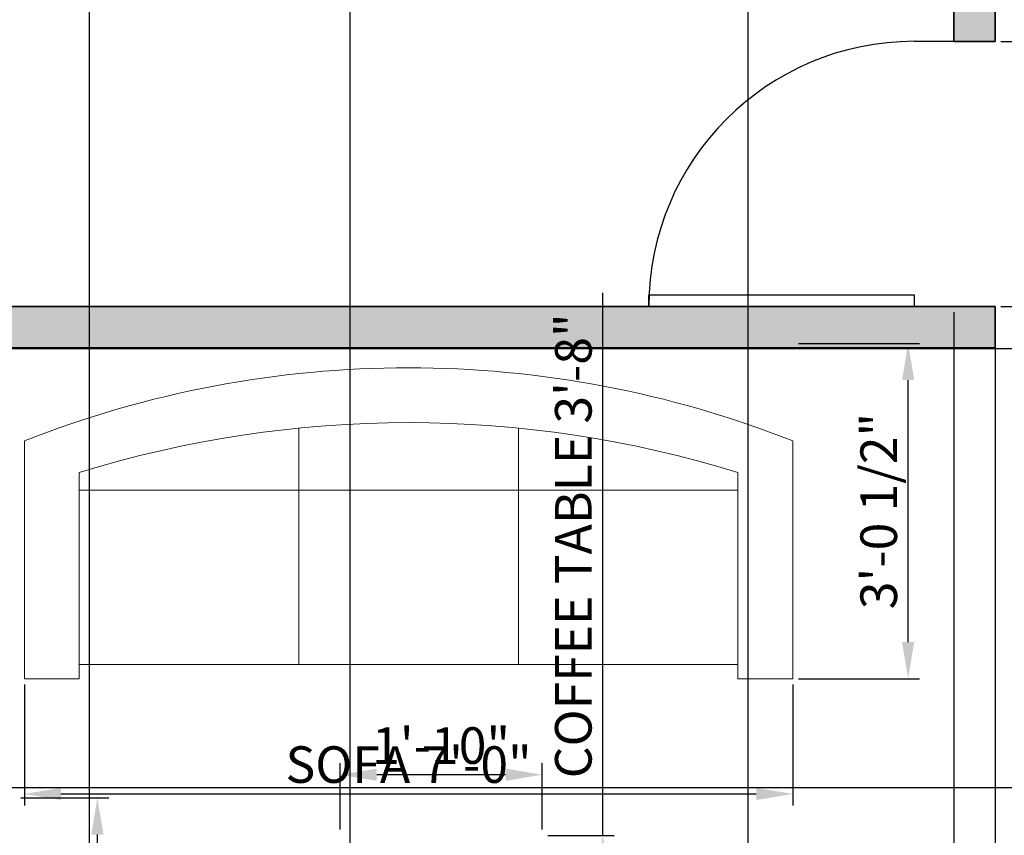
# Model space of a CAD drawing. Units: inches. Extents: x 1872 to 2380, y 714 to 1327.
# Tile 6 of 9: x 1994 to 2101, y 1055 to 1144. Entities that reach past the tile are written whole.
import ezdxf

# ---------------------------------------------------------------- set-up
doc = ezdxf.new("R2010")
doc.units = ezdxf.units.IN
for name, color, linetype, lineweight in [('A-ANNO-DIMS', 2, 'Continuous', 18), ('A-DOOR', 4, 'Continuous', 25), ('A-FURN', 8, 'Continuous', 18), ('A-WALL', 7, 'Continuous', 35)]:
    doc.layers.add(name, color=color, linetype=linetype, lineweight=lineweight)
doc.layers.add('A-WALL-PATT', color=242, linetype='Continuous', lineweight=13, true_color=0xd52e31)
doc.styles.get("Standard").update_dxf_attribs({"font": 'arial.ttf'})
doc.dimstyles.new('ISO-25', dxfattribs={"dimtxt": 4, "dimasz": 4, "dimexe": 1.25, "dimexo": 0.625, "dimtad": 1, "dimdec": 0, "dimlunit": 3, "dimtxsty": 'Standard', "dimcen": 2.5, "dimadec": 0, "dimazin": 0, "dimtfac": 1, "dimtdec": 0, "dimtmove": 0, "dimatfit": 3, "dimfxl": 1, "dimarcsym": 0})

# ---------------------------------------------------------------- blocks, each defined once
blk = doc.blocks.new('*U3')
for p, q in [((0, 0), (0, -6)), ((40, 0), (40, -6))]:
    blk.add_line(p, q)
blk.add_lwpolyline([(0, 0), (0, 40), (1.75, 40), (1.75, 0)], close=True)
blk.add_arc((0, 0), 40, 0, 90)
blk = doc.blocks.new('Sofa - Roundback 7 ft.')
for p, q in [((-12.00002, -32.4421), (-12.00003, -6.5971)), ((11.99997, -32.4421), (11.99998, -6.5971)), ((-36.000027, -34), (-36.000027, -11.4696)), ((35.99998, -34), (35.99998, -11.4696)), ((-35.999844, -13.3819), (35.9998, -13.3819)), ((-36.000027, -32.4421), (35.99998, -32.4421))]:
    blk.add_line(p, q)
for points in [[(-36.000027, -34), (-42.000027, -34), (-42.000027, -8)], [(41.99998, -8), (41.99998, -34), (35.99998, -34)]]:
    blk.add_lwpolyline(points)
for centre, radius, start, end in [((0, -114.25), 114.25, 68.43141, 111.5686), ((-0.00001, -127.1968), 121.1968, 72.72033, 107.2797)]:
    blk.add_arc(centre, radius, start, end)
blk = doc.blocks.new('*D40')
at = {"layer": 'A-ANNO-DIMS', "color": 0, "lineweight": -2, "transparency": 16777216}
for p, q in [((1993.9, 1059.04), (2003.52, 1059.04)), ((2002.27, 1003.04), (2002.27, 1055.04)), ((1993.9, 999.04), (2003.52, 999.04))]:
    blk.add_line(p, q, dxfattribs=at)
at = {"layer": 'A-ANNO-DIMS', "color": 0, "transparency": 16777216}
for points in [[(2001.61, 1055.04), (2002.94, 1055.04), (2002.27, 1059.04)], [(2001.61, 1003.04), (2002.94, 1003.04), (2002.27, 999.04)]]:
    blk.add_solid(points, dxfattribs=at)
at = {"layer": 'Defpoints', "color": 0, "transparency": 16777216}
for p in [(1993.27, 1059.04), (2002.27, 1059.04), (1993.27, 999.04)]:
    blk.add_point(p, dxfattribs=at)
at = {"layer": 'A-ANNO-DIMS', "color": 0, "transparency": 16777216, "insert": (1999.58, 1029.04), "char_height": 4, "attachment_point": 5, "rotation": 90}
blk.add_mtext('LOVESEAT 5\'-0"', dxfattribs=at)
blk = doc.blocks.new('*D42')
at = {"layer": 'A-ANNO-DIMS', "color": 0, "lineweight": -2, "transparency": 16777216}
for p, q in [((1994.29, 1071.45), (1994.29, 1058.23)), ((2078.29, 1071.45), (2078.29, 1058.23)), ((1998.29, 1059.48), (2074.29, 1059.48))]:
    blk.add_line(p, q, dxfattribs=at)
at = {"layer": 'A-ANNO-DIMS', "color": 0, "transparency": 16777216}
for points in [[(1998.29, 1060.14), (1998.29, 1058.81), (1994.29, 1059.48)], [(2074.29, 1060.14), (2074.29, 1058.81), (2078.29, 1059.48)]]:
    blk.add_solid(points, dxfattribs=at)
at = {"layer": 'Defpoints', "color": 0, "transparency": 16777216}
for p in [(1994.29, 1072.08), (2078.29, 1072.08), (2078.29, 1059.48)]:
    blk.add_point(p, dxfattribs=at)
at = {"layer": 'A-ANNO-DIMS', "color": 0, "transparency": 16777216, "insert": (2036.29, 1062.17), "char_height": 4, "attachment_point": 5}
blk.add_mtext('SOFA 7\'-0"', dxfattribs=at)
blk = doc.blocks.new('*D43')
at = {"layer": 'A-ANNO-DIMS', "color": 0, "lineweight": -2, "transparency": 16777216}
for p, q in [((2078.91, 1108.74), (2092.14, 1108.74)), ((2090.89, 1076.08), (2090.89, 1104.74)), ((2078.91, 1072.08), (2092.14, 1072.08))]:
    blk.add_line(p, q, dxfattribs=at)
at = {"layer": 'A-ANNO-DIMS', "color": 0, "transparency": 16777216}
for points in [[(2090.22, 1104.74), (2091.55, 1104.74), (2090.89, 1108.74)], [(2090.22, 1076.08), (2091.55, 1076.08), (2090.89, 1072.08)]]:
    blk.add_solid(points, dxfattribs=at)
at = {"layer": 'Defpoints', "color": 0, "transparency": 16777216}
for p in [(2078.29, 1108.74), (2090.89, 1108.74), (2078.29, 1072.08)]:
    blk.add_point(p, dxfattribs=at)
at = {"layer": 'A-ANNO-DIMS', "color": 0, "transparency": 16777216, "insert": (2088.19, 1090.41), "char_height": 4, "attachment_point": 5, "rotation": 90}
blk.add_mtext('3\'-0 1/2"', dxfattribs=at)
blk = doc.blocks.new('*D44')
at = {"layer": 'A-ANNO-DIMS', "color": 0, "lineweight": -2, "transparency": 16777216}
for p, q in [((2057.51, 1054.95), (2057.51, 1114.26)), ((2051.51, 1054.95), (2058.76, 1054.95)), ((2057.51, 1014.78), (2057.51, 1050.95)), ((2051.51, 1010.78), (2058.76, 1010.78))]:
    blk.add_line(p, q, dxfattribs=at)
at = {"layer": 'A-ANNO-DIMS', "color": 0, "transparency": 16777216}
for points in [[(2056.84, 1050.95), (2058.17, 1050.95), (2057.51, 1054.95)], [(2056.84, 1014.78), (2058.17, 1014.78), (2057.51, 1010.78)]]:
    blk.add_solid(points, dxfattribs=at)
at = {"layer": 'Defpoints', "color": 0, "transparency": 16777216}
for p in [(2050.88, 1054.95), (2057.51, 1054.95), (2050.88, 1010.78)]:
    blk.add_point(p, dxfattribs=at)
at = {"layer": 'A-ANNO-DIMS', "color": 0, "transparency": 16777216, "insert": (2054.81, 1086.61), "char_height": 4, "attachment_point": 5, "rotation": 90}
blk.add_mtext('COFFEE TABLE 3\'-8"', dxfattribs=at)
blk = doc.blocks.new('*D45')
at = {"layer": 'A-ANNO-DIMS', "color": 0, "lineweight": -2, "transparency": 16777216}
for p, q in [((2028.8, 1055.58), (2028.8, 1062.83)), ((2050.88, 1055.58), (2050.88, 1062.83)), ((2046.88, 1061.58), (2032.8, 1061.58))]:
    blk.add_line(p, q, dxfattribs=at)
at = {"layer": 'A-ANNO-DIMS', "color": 0, "transparency": 16777216}
for points in [[(2032.8, 1062.25), (2032.8, 1060.91), (2028.8, 1061.58)], [(2046.88, 1062.25), (2046.88, 1060.91), (2050.88, 1061.58)]]:
    blk.add_solid(points, dxfattribs=at)
at = {"layer": 'Defpoints', "color": 0, "transparency": 16777216}
for p in [(2028.8, 1061.58), (2028.8, 1054.95), (2050.88, 1054.95)]:
    blk.add_point(p, dxfattribs=at)
at = {"layer": 'A-ANNO-DIMS', "color": 0, "transparency": 16777216, "insert": (2039.84, 1064.25), "char_height": 4, "attachment_point": 5}
blk.add_mtext('1\'-10"', dxfattribs=at)
blk = doc.blocks.new('*D67')
at = {"layer": 'A-ANNO-DIMS', "color": 0, "lineweight": -2, "transparency": 16777216}
for p, q in [((1943.77, 1112.77), (1905.35, 1112.77)), ((1906.6, 956.99), (1906.6, 1108.77)), ((2000.77, 952.99), (1905.35, 952.99))]:
    blk.add_line(p, q, dxfattribs=at)
at = {"layer": 'A-ANNO-DIMS', "color": 0, "transparency": 16777216}
for points in [[(1905.93, 1108.77), (1907.27, 1108.77), (1906.6, 1112.77)], [(1905.93, 956.99), (1907.27, 956.99), (1906.6, 952.99)]]:
    blk.add_solid(points, dxfattribs=at)
at = {"layer": 'Defpoints', "color": 0, "transparency": 16777216}
for p in [(1906.6, 1112.77), (1944.4, 1112.77), (2001.4, 952.99)]:
    blk.add_point(p, dxfattribs=at)
at = {"layer": 'A-ANNO-DIMS', "color": 0, "transparency": 16777216, "insert": (1903.93, 1032.88), "char_height": 4, "attachment_point": 5, "rotation": 90}
blk.add_mtext('13\'-4"', dxfattribs=at)
blk = doc.blocks.new('*D69')
at = {"layer": 'A-ANNO-DIMS', "color": 0, "lineweight": -2, "transparency": 16777216}
for p, q in [((2101.02, 1141.77), (2377.6, 1141.77)), ((2376.35, 1116.77), (2376.35, 1137.77)), ((2101.02, 1112.77), (2377.6, 1112.77))]:
    blk.add_line(p, q, dxfattribs=at)
at = {"layer": 'A-ANNO-DIMS', "color": 0, "transparency": 16777216}
for points in [[(2375.68, 1137.77), (2377.01, 1137.77), (2376.35, 1141.77)], [(2375.68, 1116.77), (2377.01, 1116.77), (2376.35, 1112.77)]]:
    blk.add_solid(points, dxfattribs=at)
at = {"layer": 'Defpoints', "color": 0, "transparency": 16777216}
for p in [(2100.4, 1141.77), (2376.35, 1141.77), (2100.4, 1112.77)]:
    blk.add_point(p, dxfattribs=at)
at = {"layer": 'A-ANNO-DIMS', "color": 0, "transparency": 16777216, "insert": (2373.68, 1127.27), "char_height": 4, "attachment_point": 5, "rotation": 90}
blk.add_mtext('2\'-5"', dxfattribs=at)
blk = doc.blocks.new('*D72')
at = {"layer": 'A-ANNO-DIMS', "color": 0, "lineweight": -2, "transparency": 16777216}
for p, q in [((2197.27, 1108.14), (1905.35, 1108.14)), ((1906.6, 1064.14), (1906.6, 1104.14)), ((2197.27, 1060.14), (1905.35, 1060.14))]:
    blk.add_line(p, q, dxfattribs=at)
at = {"layer": 'A-ANNO-DIMS', "color": 0, "transparency": 16777216}
for points in [[(1905.93, 1104.14), (1907.27, 1104.14), (1906.6, 1108.14)], [(1905.93, 1064.14), (1907.27, 1064.14), (1906.6, 1060.14)]]:
    blk.add_solid(points, dxfattribs=at)
at = {"layer": 'Defpoints', "color": 0, "transparency": 16777216}
for p in [(1906.6, 1108.14), (2197.9, 1108.14), (2197.9, 1060.14)]:
    blk.add_point(p, dxfattribs=at)
at = {"layer": 'A-ANNO-DIMS', "color": 0, "transparency": 16777216, "insert": (1903.93, 1084.14), "char_height": 4, "attachment_point": 5, "rotation": 90}
blk.add_mtext('4\'-0"', dxfattribs=at)
blk = doc.blocks.new('*D76')
at = {"layer": 'A-ANNO-DIMS', "color": 0, "lineweight": -2, "transparency": 16777216}
for p, q in [((2001.4, 953.62), (2001.4, 1319.69)), ((2029.9, 953.62), (2029.9, 1319.69)), ((2005.4, 1318.44), (2025.9, 1318.44))]:
    blk.add_line(p, q, dxfattribs=at)
at = {"layer": 'A-ANNO-DIMS', "color": 0, "transparency": 16777216}
for points in [[(2005.4, 1319.11), (2005.4, 1317.78), (2001.4, 1318.44)], [(2025.9, 1319.11), (2025.9, 1317.78), (2029.9, 1318.44)]]:
    blk.add_solid(points, dxfattribs=at)
at = {"layer": 'Defpoints', "color": 0, "transparency": 16777216}
for p in [(2029.9, 1318.44), (2001.4, 952.99), (2029.9, 952.99)]:
    blk.add_point(p, dxfattribs=at)
at = {"layer": 'A-ANNO-DIMS', "color": 0, "transparency": 16777216, "insert": (2015.65, 1321.14), "char_height": 4, "attachment_point": 5}
blk.add_mtext('2\'-4 1/2"', dxfattribs=at)
blk = doc.blocks.new('*D77')
at = {"layer": 'A-ANNO-DIMS', "color": 0, "lineweight": -2, "transparency": 16777216}
for p, q in [((2029.9, 953.62), (2029.9, 1319.69)), ((2073.4, 953.62), (2073.4, 1319.69)), ((2033.9, 1318.44), (2069.4, 1318.44))]:
    blk.add_line(p, q, dxfattribs=at)
at = {"layer": 'A-ANNO-DIMS', "color": 0, "transparency": 16777216}
for points in [[(2033.9, 1319.11), (2033.9, 1317.78), (2029.9, 1318.44)], [(2069.4, 1319.11), (2069.4, 1317.78), (2073.4, 1318.44)]]:
    blk.add_solid(points, dxfattribs=at)
at = {"layer": 'Defpoints', "color": 0, "transparency": 16777216}
for p in [(2073.4, 1318.44), (2029.9, 952.99), (2073.4, 952.99)]:
    blk.add_point(p, dxfattribs=at)
at = {"layer": 'A-ANNO-DIMS', "color": 0, "transparency": 16777216, "insert": (2051.65, 1321.14), "char_height": 4, "attachment_point": 5}
blk.add_mtext('3\'-7 1/2"', dxfattribs=at)
blk = doc.blocks.new('*D80')
at = {"layer": 'A-ANNO-DIMS', "color": 0, "lineweight": -2, "transparency": 16777216}
for p, q in [((2095.9, 1112.15), (2095.9, 716.39)), ((2100.4, 1112.15), (2100.4, 716.39)), ((2091.9, 717.64), (2087.9, 717.64)), ((2095.9, 717.64), (2100.4, 717.64)), ((2104.4, 717.64), (2129.6, 717.64))]:
    blk.add_line(p, q, dxfattribs=at)
at = {"layer": 'A-ANNO-DIMS', "color": 0, "transparency": 16777216}
for points in [[(2091.9, 718.3), (2091.9, 716.97), (2095.9, 717.64)], [(2104.4, 718.3), (2104.4, 716.97), (2100.4, 717.64)]]:
    blk.add_solid(points, dxfattribs=at)
at = {"layer": 'Defpoints', "color": 0, "transparency": 16777216}
for p in [(2095.9, 1112.77), (2100.4, 1112.77), (2100.4, 717.64)]:
    blk.add_point(p, dxfattribs=at)
at = {"layer": 'A-ANNO-DIMS', "color": 0, "transparency": 16777216, "insert": (2119, 720.33), "char_height": 4, "attachment_point": 5}
blk.add_mtext('0\'-4 1/2"', dxfattribs=at)

msp = doc.modelspace()

# ---------------------------------------------------------------- hatches: boundary and pattern name
at = {"layer": 'A-WALL-PATT', "transparency": 33554687}
h = msp.add_hatch(color=256, dxfattribs=at)
h.dxf.hatch_style = 1
h.paths.add_polyline_path([(2295.4, 1289.64), (1935.4, 1289.64), (1935.4, 809.64), (1949.4, 809.64), (1949.4, 818.64), (1944.4, 818.64), (1944.4, 1108.27), (2100.4, 1108.27), (2100.4, 1112.77), (1944.4, 1112.77), (1944.4, 1280.64), (2095.9, 1280.64), (2095.9, 1141.77), (2100.4, 1141.77), (2100.4, 1280.64), (2169.91, 1280.64), (2169.91, 1244.64), (2169.91, 1160.49, -0.053008), (2170.04, 1158.75, -0.03687), (2169.91, 1157.54), (2169.91, 1148.64), (2167.91, 1148.64), (2138.4, 1148.64), (2138.4, 1144.14), (2167.91, 1144.14), (2174.41, 1144.14), (2174.41, 1280.64), (2197.9, 1280.64), (2197.9, 1184.64), (2202.4, 1184.64), (2202.4, 1280.64), (2286.4, 1280.64), (2286.4, 1148.64), (2197.9, 1148.64), (2197.9, 1108.14), (2202.4, 1108.14), (2202.4, 1144.14), (2286.4, 1144.14), (2286.4, 1060.14), (2202.4, 1060.14), (2202.4, 1108.14), (2197.9, 1108.14), (2197.9, 1060.14), (2197.9, 1053.64), (2202.4, 1053.64), (2202.4, 1055.64), (2286.4, 1055.64), (2286.4, 976.14), (2202.4, 976.14), (2202.4, 1015.64), (2197.9, 1015.64), (2197.9, 971.64), (2197.9, 952.99), (2197.9, 818.64), (2101.9, 818.64), (2101.9, 948.71), (2130.4, 948.71), (2130.4, 952.99), (2073.4, 952.99), (2073.4, 948.71), (2097.4, 948.71), (2097.4, 818.64), (2005.9, 818.64), (2005.9, 948.71), (2029.9, 948.71), (2029.9, 952.99), (2001.4, 952.99), (2001.4, 818.64), (1996.4, 818.64), (1985.23, 818.64), (1985.23, 809.64), (1996.4, 809.64), (2295.4, 809.64)])
h.paths.add_polyline_path([(2202.4, 971.64), (2286.4, 971.64), (2286.4, 858.19), (2286.62, 858.19), (2286.62, 857.19), (2286.4, 857.19), (2286.4, 828.68), (2286.48, 828.76), (2286.4, 828.43), (2286.4, 818.64), (2256.29, 818.64), (2255.29, 818.39), (2254.54, 818.64), (2238.99, 818.64), (2238.75, 818.58), (2238.56, 818.64), (2202.4, 818.64), (2202.4, 952.99)], flags=16)
h.paths.add_polyline_path([(2260.41, 970, -0.15), (2280.41, 970), (2278.41, 967, 0.001913), (2277.92, 967.06), (2277.41, 964.5), (2278.64, 964.5), (2278.72, 964), (2279.41, 964), (2282.41, 953, -0.541163), (2280.76, 950.93), (2280.91, 950, -0.414214), (2279.91, 949), (2279.41, 949), (2279.91, 945), (2278.41, 945), (2277.91, 949), (2270.41, 949), (2262.91, 949), (2262.41, 945), (2260.91, 945), (2261.41, 949), (2260.91, 949, -0.414214), (2259.91, 950), (2260.05, 950.93, -0.505809), (2258.36, 952.83), (2261.41, 964), (2262.1, 964), (2262.17, 964.5), (2263.41, 964.5), (2262.9, 967.06, 0.001913), (2262.41, 967)], flags=0)
h.paths.add_polyline_path([(2257.85, 934.42), (2280.51, 934.42, -0.333333), (2281.77, 933.16), (2281.77, 923.09, -0.333333), (2280.51, 921.83), (2277.57, 921.83), (2277.57, 921.41), (2275.89, 921.41), (2275.89, 921.83), (2262.46, 921.83), (2262.46, 921.41), (2260.79, 921.41), (2260.79, 921.83), (2257.85, 921.83, -0.333333), (2256.59, 923.09), (2256.59, 933.16, -0.333333)], flags=0)
h.paths.add_polyline_path([(2260.61, 912.79), (2262.11, 912.79), (2262.61, 908.79), (2270.11, 908.79), (2277.61, 908.79), (2278.11, 912.79), (2279.61, 912.79), (2279.11, 908.79), (2279.61, 908.79, -0.414214), (2280.61, 907.79), (2280.46, 906.86, -0.505809), (2282.15, 904.96), (2279.11, 893.79), (2278.42, 893.79), (2278.34, 893.29), (2277.11, 893.29), (2277.62, 890.73, 0.001913), (2278.11, 890.79), (2280.11, 887.79, -0.15), (2260.11, 887.79), (2262.11, 890.79, 0.001913), (2262.59, 890.73), (2263.11, 893.29), (2261.87, 893.29), (2261.79, 893.79), (2261.11, 893.79), (2258.11, 904.79, -0.541163), (2259.75, 906.86), (2259.61, 907.79, -0.414214), (2260.61, 908.79), (2261.11, 908.79)], flags=0)
h.paths.add_polyline_path([(2252.62, 864.69), (2253.62, 864.69), (2253.62, 862.19), (2253.62, 860.69), (2256.62, 859.69, -0.362186), (2259.62, 862.19, -0.174416), (2262.62, 860.69, 0.103487), (2265.62, 859.19, -0.219276), (2266.55, 858.19), (2268.62, 858.19), (2268.62, 859.69), (2267.62, 859.69), (2267.62, 863.69), (2270.12, 863.69), (2270.12, 859.69), (2269.12, 859.69), (2269.12, 858.19), (2274.62, 858.19), (2278.62, 858.19), (2278.62, 862.69), (2275.62, 864.69), (2275.62, 865.69), (2279.62, 862.69), (2279.62, 858.19), (2279.62, 852.69), (2275.62, 849.19), (2275.62, 850.19), (2278.62, 852.69), (2278.62, 857.19), (2274.62, 857.19), (2271.12, 857.19), (2271.12, 855.69), (2272.12, 855.69), (2272.12, 851.69), (2269.62, 851.69), (2269.62, 855.69), (2270.62, 855.69), (2270.62, 857.19), (2266.55, 857.19, -0.219162), (2265.62, 856.19, 0.103506), (2262.62, 854.69, -0.174459), (2259.62, 853.19, -0.362114), (2256.62, 855.69), (2253.62, 854.69), (2253.62, 850.69), (2252.62, 850.69)], flags=0)
h.paths.add_polyline_path([(2253.62, 859.69), (2256.62, 858.69), (2256.62, 856.69), (2253.62, 855.69)], flags=0)
h.paths.add_polyline_path([(2208.62, 838.17), (2208.28, 836.61), (2207.75, 836.18), (2207.67, 833.93), (2208.71, 832.96), (2211.55, 836.09), (2214.43, 837.53), (2214.45, 837.55), (2214.61, 836.16), (2215.48, 834.9), (2215.87, 835.13), (2217.12, 836.79), (2216.83, 834.17), (2218.8, 828.76), (2219.23, 829.13), (2220.06, 831.53), (2219.5, 837.61), (2219.53, 837.66), (2219.68, 838.72), (2219.62, 838.91), (2219.72, 839.01), (2219.51, 837.47), (2219.77, 834.68), (2220.87, 834.05), (2221.03, 834.58), (2222.05, 835.47), (2222.71, 834.65), (2223.67, 836.89), (2224.63, 836.57), (2226.23, 835.08), (2227.55, 836.18), (2227.59, 837.16), (2228.42, 838.17), (2228.08, 836.61), (2227.55, 836.18), (2227.47, 833.93), (2228.51, 832.96), (2231.35, 836.09), (2234.23, 837.53), (2234.25, 837.55), (2234.42, 836.16), (2235.28, 834.9), (2235.67, 835.13), (2236.93, 836.79), (2236.93, 836.84), (2238.69, 834.65), (2239.41, 836.34), (2239.3, 837.61), (2239.34, 837.66), (2239.48, 838.72), (2239.42, 838.91), (2239.52, 839.01), (2239.31, 837.47), (2239.36, 836.98), (2240.61, 836.57), (2242.2, 835.08), (2243.53, 836.18), (2243.57, 837.16), (2244.39, 838.17), (2244.05, 836.61), (2243.53, 836.18), (2243.44, 833.93), (2244.49, 832.96), (2247.33, 836.09), (2250.21, 837.53), (2250.22, 837.55), (2250.39, 836.16), (2251.25, 834.9), (2251.65, 835.13), (2252.9, 836.79), (2252.61, 834.17), (2254.09, 830.08), (2254.54, 829.37), (2254.85, 828.99), (2255.01, 829.13), (2255.83, 831.53), (2255.29, 837.44), (2255.28, 837.44), (2255.46, 838.72), (2255.4, 838.91), (2255.5, 839.01), (2255.28, 837.47), (2255.29, 837.44), (2257.9, 836.57), (2259.5, 835.08), (2260.82, 836.18), (2260.86, 837.16), (2261.69, 838.17), (2261.35, 836.61), (2260.82, 836.18), (2260.74, 833.93), (2261.78, 832.96), (2264.62, 836.09), (2267.5, 837.53), (2267.52, 837.55), (2267.68, 836.16), (2268.54, 834.9), (2268.94, 835.13), (2270.19, 836.79), (2269.9, 834.17), (2271.79, 828.96), (2271.98, 828.86), (2272.3, 829.13), (2273.13, 831.53), (2272.56, 837.61), (2272.6, 837.66), (2272.75, 838.72), (2272.69, 838.91), (2272.79, 839.01), (2272.58, 837.47), (2273.13, 831.53), (2273.02, 831.22), (2273.67, 831.01), (2273.92, 831.6), (2273.83, 830.95), (2274.1, 830.86), (2275.75, 833.35), (2276.03, 831.86), (2276.57, 831.38), (2277, 831.91), (2277.3, 833.27), (2279.06, 830.44), (2281.09, 831.46), (2281.1, 831.48), (2281.21, 830.5), (2281.82, 829.61), (2282.1, 829.77), (2282.98, 830.94), (2282.77, 829.1), (2284.15, 825.3), (2284.46, 825.55), (2285.04, 827.24), (2284.64, 831.51), (2284.67, 831.55), (2284.77, 832.3), (2284.73, 832.43), (2284.8, 832.5), (2284.65, 831.42), (2285.04, 827.24), (2284.46, 825.55), (2283.45, 824.71), (2281.76, 819.99), (2278.73, 818.64), (2276.7, 819.65), (2275.69, 821.34), (2274.34, 822.01), (2272.32, 824.04), (2269.58, 824.33), (2268.46, 821.21), (2264.14, 819.29), (2261.26, 820.73), (2259.82, 823.13), (2257.9, 824.09), (2255.02, 826.97), (2253.29, 827.15), (2251.17, 821.21), (2246.85, 819.29), (2243.97, 820.73), (2242.53, 823.13), (2240.61, 824.09), (2237.73, 826.97), (2237.27, 827.01), (2235.19, 821.21), (2230.87, 819.29), (2227.99, 820.73), (2226.55, 823.13), (2224.63, 824.09), (2221.75, 826.97), (2217.61, 827.41), (2215.39, 821.21), (2211.07, 819.29), (2208.19, 820.73), (2206.75, 823.13), (2204.83, 824.09), (2203.87, 826.49), (2202.91, 830.81), (2202.91, 834.65), (2203.87, 836.89), (2204.83, 836.57), (2206.43, 835.08), (2207.75, 836.18), (2207.79, 837.16)], flags=0)
h.paths.add_polyline_path([(2221.04, 832.88), (2221.82, 832.52), (2222.11, 833.69), (2222.71, 834.29), (2222.71, 832.11), (2225.59, 830.81), (2226.55, 830.81), (2228.95, 822.65), (2230.87, 820.25), (2230.87, 819.29), (2233.27, 821.21), (2233.75, 823.61), (2232.79, 826.97), (2231.99, 830.19), (2236.41, 827.71), (2236.63, 831.29), (2235.93, 834.58), (2242.53, 830.81), (2241.57, 830.81), (2240.97, 831.07), (2240.47, 830.33), (2239.06, 829.14), (2239.65, 826.49), (2237.25, 829.37), (2236.52, 829.55), (2236.41, 827.71), (2231.99, 830.19), (2232.79, 826.97), (2233.75, 823.61), (2233.27, 821.21), (2230.87, 819.29), (2230.87, 820.25), (2228.95, 822.65), (2226.55, 830.81), (2225.59, 830.81), (2222.71, 832.11), (2222.71, 830.81), (2223.67, 826.49), (2221.27, 829.37), (2220.67, 830.33), (2220.67, 830.33)], flags=0)
h.paths.add_polyline_path([(2255.98, 833), (2259.82, 830.81), (2258.86, 830.81), (2257.25, 831.54), (2256.45, 830.33), (2256.66, 831.81), (2256.02, 832.1), (2255.98, 831.99)], flags=0)
h.paths.add_polyline_path([(2275.69, 826.73), (2277.07, 828.25), (2275.46, 829.74), (2276.39, 830.51), (2276.33, 828.93), (2279.06, 826.4), (2278.73, 823.36), (2277.38, 821)], flags=0)
h.paths.add_polyline_path([(2260.6, 925.25), (2276.34, 925.25), (2276.34, 931.01), (2260.6, 931.01)], flags=8)
h.paths.add_polyline_path([(2202.72, 1070.05), (2202.72, 1092.72), (2197.34, 1092.72), (2197.34, 1070.05)], flags=25)

# ---------------------------------------------------------------- linework, layer by layer
at = {"layer": 'A-WALL'}
for p, q in [((2095.9, 1141.77), (2095.9, 1280.64)), ((2100.4, 1141.77), (2100.4, 1280.64)), ((2095.9, 1141.77), (2100.4, 1141.77)), ((1944.4, 1112.77), (2100.4, 1112.77)), ((2100.4, 1108.27), (2100.4, 1112.77)), ((1944.4, 1108.27), (2100.4, 1108.27))]:
    msp.add_line(p, q, dxfattribs=at)

# ---------------------------------------------------------------- block references
at = {"layer": 'A-DOOR', "xscale": 0.7251209378833331, "yscale": 0.7251209378833331, "zscale": 0.7251209378833331, "rotation": 90}
msp.add_blockref('*U3', (2091.55, 1112.77), dxfattribs=at)
at = {"layer": 'A-FURN', "transparency": 33554687}
msp.add_blockref('Sofa - Roundback 7 ft.', (2036.29, 1106.08), dxfattribs=at)

# ---------------------------------------------------------------- dimensions: what is measured, and where the dimension line sits
at = {"layer": 'A-ANNO-DIMS', "transparency": 33554687}
for base, p1, p2, picture, middle in [((2029.9, 1318.44), (2001.4, 952.99), (2029.9, 952.99), '*D76', (2015.65, 1321.14)), ((2073.4, 1318.44), (2029.9, 952.99), (2073.4, 952.99), '*D77', (2051.65, 1321.14)), ((2100.4, 717.64), (2095.9, 1112.77), (2100.4, 1112.77), '*D80', (2119, 720.33))]:
    dim = msp.add_linear_dim(base=base, p1=p1, p2=p2, dimstyle='ISO-25', override={"dimdec": 1, "dimlfac": 1, "dimrnd": 0, "dimzin": 1, "dimdsep": 46, "dimlunit": 4, "dimfrac": 2}, dxfattribs=at)
    dim.commit()
    dim.dimension.update_dxf_attribs({"geometry": picture, "text_midpoint": middle})
for base, p1, p2, angle, picture, middle in [((2376.35, 1141.77), (2100.4, 1112.77), (2100.4, 1141.77), 90, '*D69', (2373.68, 1127.27)), ((1906.6, 1112.77), (2001.4, 952.99), (1944.4, 1112.77), 90, '*D67', (1903.93, 1032.88)), ((2090.89, 1108.74), (2078.29, 1072.08), (2078.29, 1108.74), 90, '*D43', (2088.19, 1090.41)), ((1906.6, 1108.14), (2197.9, 1060.14), (2197.9, 1108.14), 90, '*D72', (1903.93, 1084.14)), ((2028.8, 1061.58), (2050.88, 1054.95), (2028.8, 1054.95), 180, '*D45', (2039.84, 1064.25))]:
    dim = msp.add_linear_dim(base=base, p1=p1, p2=p2, angle=angle, dimstyle='ISO-25', override={"dimdec": 1, "dimlfac": 1, "dimrnd": 0, "dimzin": 1, "dimdsep": 46, "dimlunit": 4, "dimfrac": 2}, dxfattribs=at)
    dim.commit()
    dim.dimension.update_dxf_attribs({"geometry": picture, "text_midpoint": middle})
for base, p1, p2, text, picture, middle in [((2057.51, 1054.95), (2050.88, 1010.78), (2050.88, 1054.95), 'COFFEE TABLE <>', '*D44', (2054.81, 1086.61)), ((2002.27, 1059.04), (1993.27, 999.04), (1993.27, 1059.04), 'LOVESEAT <>', '*D40', (1999.58, 1029.04))]:
    dim = msp.add_linear_dim(base=base, p1=p1, p2=p2, angle=90, text=text, dimstyle='ISO-25', override={"dimdec": 1, "dimlfac": 1, "dimrnd": 0, "dimzin": 1, "dimdsep": 46, "dimlunit": 4, "dimfrac": 2}, dxfattribs=at)
    dim.commit()
    dim.dimension.update_dxf_attribs({"geometry": picture, "text_midpoint": middle})
dim = msp.add_linear_dim(base=(2078.29, 1059.48), p1=(1994.29, 1072.08), p2=(2078.29, 1072.08), text='SOFA <>', dimstyle='ISO-25', override={"dimdec": 1, "dimlfac": 1, "dimrnd": 0, "dimzin": 1, "dimdsep": 46, "dimlunit": 4, "dimfrac": 2}, dxfattribs=at)
dim.commit()
dim.dimension.update_dxf_attribs({"geometry": '*D42', "text_midpoint": (2036.29, 1062.17)})

doc.saveas('drawing.dxf')
